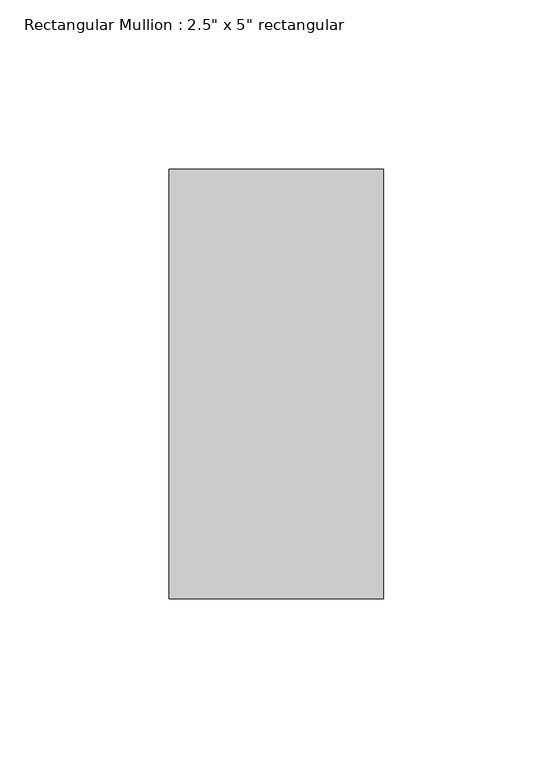
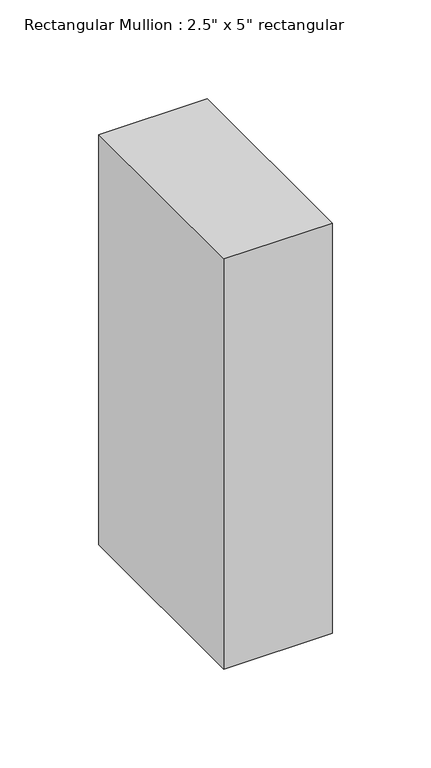
"""IFC4 building model written with IfcOpenShell, lengths in millimetres: member geometry."""

from ifc_helpers import new_model, si_unit, frame, origin, place, context, project, spatial, polyline, outline, extrude, source, transform, mapped, element, save


def member_e59d5788(model_context):
    return source(origin(), model_context, "Body", "SweptSolid", [
        extrude(outline(polyline([(31.75, 63.5), (31.75, -63.5), (-31.75, -63.5), (-31.75, 63.5), (31.75, 63.5)])), frame((0.0, 0.0, -254.0), z_axis=(0.0, 0.0, 1.0), x_axis=(1.0, 0.0, 0.0)), (0.0, 0.0, 1.0), 254.0),
    ])


if __name__ == "__main__":
    model = new_model("IFC4")
    model_context = context("Model", 3, world=origin())
    ifc_project = project(units=[si_unit("LENGTHUNIT", "METRE", prefix="MILLI")], contexts=[model_context])
    site = spatial("IfcSite", under=ifc_project)
    building = spatial("IfcBuilding", under=site)
    placement = place(None, origin())
    member_shape = member_e59d5788(model_context)
    element("IfcMember", 1, ObjectType="Rectangular Mullion : 2.5\" x 5\" rectangular", at=placement, inside=building, context=model_context, shape_type="MappedRepresentation", body=[
        mapped(member_shape, transform((0.0, 0.0, 0.0), x_axis=(1.0, 0.0, 0.0), y_axis=(0.0, 1.0, 0.0), z_axis=(0.0, 0.0, 1.0))),
    ])
    save(model, "model.ifc")

# Revit data of these elements
# Type "Rectangular Mullion : 2.5\" x 5\" rectangular"
#   built-in parameter 1007304 = 0.416667 (stored number, unit not read)
#   built-in parameter 1007301 = 0.104167 (stored number, unit not read)
#   built-in parameter 1007300 = 0.104167 (stored number, unit not read)
# Element 1 (IfcMember, "Rectangular Mullion : 2.5\" x 5\" rectangular")
#   Materials on its faces: "Aluminum"
# Materials
#   "Aluminum": class "Metal", colour RGB 247 247 247, transparency 0, Description = "Aluminum 6061", Cost = 0
